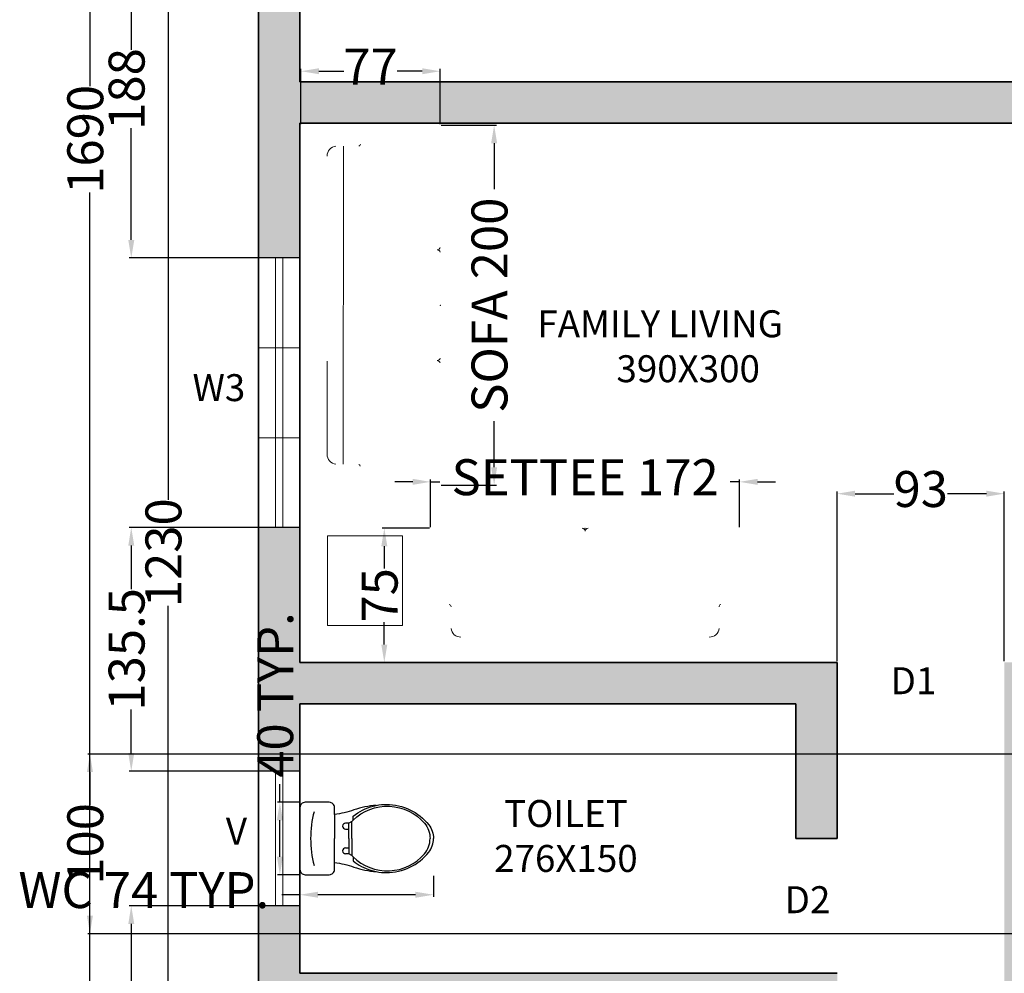
# Model space of a CAD drawing. Units: centimetres. Extents: x 2137 to 3697, y 183 to 2094.
# Tile 2 of 8: x 2137 to 2685, y 678 to 1208. Entities that reach past the tile are written whole.
import ezdxf

# ---------------------------------------------------------------- set-up
doc = ezdxf.new("R2010")
doc.units = ezdxf.units.CM
for name, color, linetype, lineweight in [('A-ANNO-DIMS', 2, 'Continuous', 18), ('A-ANNO-TEXT', 7, 'Continuous', 18), ('A-AREA-IDEN', 7, 'Continuous', 25), ('A-FLOR-FIXT', 71, 'Continuous', 18), ('A-FURN', 8, 'Continuous', 18), ('A-GLAZ', 4, 'Continuous', 18), ('A-WALL', 7, 'Continuous', 35), ('A-WALL-PATT', 52, 'Continuous', 13)]:
    doc.layers.add(name, color=color, linetype=linetype, lineweight=lineweight)
doc.layers.add('WC-Detail_dwgmodels.com', color=251, linetype='Continuous')
doc.layers.add('WC-Outline_dwgmodels.com', color=250, linetype='Continuous')
doc.styles.get("Standard").update_dxf_attribs({"font": 'arial.ttf'})
doc.dimstyles.new('ISO-25', dxfattribs={"dimtxt": 20, "dimasz": 10, "dimexe": 1.25, "dimexo": 0.625, "dimtad": 0, "dimtxsty": 'Standard', "dimcen": 2.5, "dimadec": 0, "dimazin": 0, "dimtfac": 1, "dimtmove": 0, "dimatfit": 3, "dimfxl": 1, "dimarcsym": 0})

# ---------------------------------------------------------------- blocks, each defined once
blk = doc.blocks.new('*D7')
at = {"layer": 'A-ANNO-DIMS', "color": 0, "lineweight": -2, "transparency": 16777216}
for p, q in [((2269.4, 1526.58), (2218.41, 1526.58)), ((2219.66, 1516.58), (2219.66, 941.09)), ((2219.66, 306.58), (2219.66, 882.07)), ((2269.4, 296.58), (2218.41, 296.58))]:
    blk.add_line(p, q, dxfattribs=at)
at = {"layer": 'A-ANNO-DIMS', "color": 0, "transparency": 16777216}
for points in [[(2217.99, 1516.58), (2221.33, 1516.58), (2219.66, 1526.58)], [(2217.99, 306.58), (2221.33, 306.58), (2219.66, 296.58)]]:
    blk.add_solid(points, dxfattribs=at)
at = {"layer": 'Defpoints', "color": 0, "transparency": 16777216}
for p in [(2270.02, 1526.58), (2219.66, 296.58), (2270.02, 296.58)]:
    blk.add_point(p, dxfattribs=at)
at = {"layer": 'A-ANNO-DIMS', "color": 0, "transparency": 16777216, "insert": (2219.66, 911.58), "char_height": 20, "attachment_point": 5, "rotation": 90}
blk.add_mtext('1230', dxfattribs=at)
blk = doc.blocks.new('PAN')
at = {"layer": 'WC-Detail_dwgmodels.com'}
for p, q in [((3002.19, 2116.71), (3003.1, 2118.39)), ((3003.1, 2118.39), (3003.1, 2120.22)), ((3006.38, 2118.39), (3003.1, 2118.39)), ((3006.38, 2120.22), (3006.38, 2118.39)), ((3011.63, 2118.39), (3006.38, 2118.39)), ((3011.63, 2118.39), (3016.89, 2118.39)), ((3016.89, 2120.22), (3016.89, 2118.39)), ((3016.89, 2118.39), (3020.16, 2118.39)), ((3020.16, 2118.39), (3020.16, 2120.22)), ((3021.08, 2116.71), (3020.16, 2118.39))]:
    blk.add_line(p, q, dxfattribs=at)
for points in [[(3001.49, 2116.03, 0.434217), (3003.1, 2076.32, 0.182634), (3011.63, 2073.2, 2.693815)], [(2999.21, 2116.03, 0.094048), (2994, 2106.21, 0.16845)], [(3001.49, 2116.03), (2999.21, 2116.03, 0.416606)], [(3002.19, 2116.71, 0.008985), (3001.49, 2116.03, 0.182634)], [(3011.63, 2116.71), (3002.19, 2116.71, 0.008985)], [(3011.63, 2116.71), (3021.08, 2116.71, -0.444938)], [(3021.78, 2116.03, -0.434217), (3020.16, 2076.32, -0.182634), (3011.63, 2073.2, -2.693815)], [(3021.08, 2116.71, -0.008985), (3021.78, 2116.03, -0.182634)], [(3021.78, 2116.03), (3024.05, 2116.03, -0.416606)], [(3024.05, 2116.03, -0.105447), (3029.64, 2104.91, -0.16845)], [(2994, 2106.21, 0.026594), (2993.22, 2103.13, 0.16845)], [(3029.64, 2104.91, -0.015301), (3030.05, 2103.13, -0.16845)]]:
    blk.add_lwpolyline(points, format="xyb", dxfattribs=at)
for centre, radius, start, end in [((3011.66, 2080.58), 59.08, 90.028, 104.6712), ((3011.6, 2080.58), 59.08, 75.3288, 89.972), ((3004.74, 2120.22), 1.64, 0, 180), ((3018.53, 2120.22), 1.64, 0, 180)]:
    blk.add_arc(centre, radius, start, end, dxfattribs=at)
at = {"layer": 'WC-Outline_dwgmodels.com'}
for points in [[(3028.88, 2126.37, 0.414214), (3031.77, 2129.26), (3031.77, 2142.74, 0.414214), (3028.88, 2145.63), (3011.63, 2145.63), (2994.39, 2145.63, 0.414214), (2991.49, 2142.74), (2991.49, 2129.26, 0.414214), (2994.39, 2126.37), (2998.34, 2126.37, -0.052345), (2995.73, 2115.59, 0.071131), (2993.22, 2103.13, 0.160777)], [(2998.34, 2126.37), (3011.63, 2126.37, 0.414214)], [(3024.93, 2126.37), (3011.63, 2126.37, -0.414214)], [(3030.05, 2103.13, 0.071131), (3027.53, 2115.59, -0.052345), (3024.93, 2126.37), (3028.88, 2126.37, 0.414214)], [(2993.22, 2103.13, 0.048023), (2992.66, 2097.45, 0.16845)], [(3030.05, 2103.13, -0.048023), (3030.61, 2097.45, -0.16845)], [(2992.66, 2097.45, 0.230343), (3004.02, 2073.95, 0.16845), (3011.63, 2071.31, 2.883082)], [(3030.61, 2097.45, -0.230343), (3019.25, 2073.95, -0.16845), (3011.63, 2071.31, -2.883082)]]:
    blk.add_lwpolyline(points, format="xyb", dxfattribs=at)
blk = doc.blocks.new('Clinicians and patient chairs 9_dwgmodels.com')
at = {"color": 0}
for points in [[(-907.9, 0, 0, 0, 0), (-959.6, -11.1, 4.62, 4.62, 0)], [(907.9, 0, 0, 0, 0), (-907.9, 0, 4.62, 4.62, 0)], [(959.6, -11.1, 0, 0, 0), (907.9, 0, 4.62, 4.62, 0)], [(-994.7, -35.9, 0, 0, 0), (-1015.6, -68.3, 4.62, 4.62, 0)], [(-959.6, -11.1, 0, 0, 0), (-994.7, -35.9, 4.62, 4.62, 0)], [(994.7, -35.9, 0, 0, 0), (959.6, -11.1, 4.62, 4.62, 0)], [(1015.6, -68.3, 0, 0, 0), (994.7, -35.9, 4.62, 4.62, 0)], [(-1015.6, -68.3, 0, 0, 0), (-1025.5, -106.3, 4.62, 4.62, 0)], [(-1025.5, -106.3, 0, 0, 0), (-1025.5, -779.5, 4.62, 4.62, 0)], [(1025.5, -106.3, 0, 0, 0), (1015.6, -68.3, 4.62, 4.62, 0)], [(1025.5, -779.5, 0, 0, 0), (1025.5, -106.3, 4.62, 4.62, 0)], [(-313.4, -149.9, 0, 0, 0), (-318.1, -149.9, 4.62, 4.62, 0)], [(-314.5, -150.4, 0, 0, 0), (-315.7, -159.3, 4.62, 4.62, 0)], [(-315.7, -159.3, 0, 0, 0), (-315.7, -777.3, 4.62, 4.62, 0)], [(-309.5, -148.3, 0, 0, 0), (-314.5, -150.4, 4.62, 4.62, 0)], [(-308, -148.3, 0, 0, 0), (-309.5, -148.3, 4.62, 4.62, 0)], [(-307.5, -148.3, 0, 0, 0), (-308, -148.3, 4.62, 4.62, 0)], [(242.9, -148.3, 0, 0, 0), (-307.5, -148.3, 4.62, 4.62, 0)], [(242.9, -148.3, 0, 0, 0), (296, -148.3, 4.62, 4.62, 0)], [(296, -148.3, 0, 0, 0), (307.5, -148.3, 4.62, 4.62, 0)], [(308, -148.3, 0, 0, 0), (307.5, -148.3, 4.62, 4.62, 0)], [(309.5, -148.3, 0, 0, 0), (308, -148.3, 4.62, 4.62, 0)], [(309.5, -148.3, 0, 0, 0), (314.5, -150.4, 4.62, 4.62, 0)], [(849.5, -149.9, 0, 0, 0), (313.4, -149.9, 4.62, 4.62, 0)], [(314.5, -150.4, 0, 0, 0), (315.7, -159.3, 4.62, 4.62, 0)], [(315.7, -159.3, 0, 0, 0), (315.7, -777.3, 4.62, 4.62, 0)], [(315.7, -161.8, 0, 0, 0), (315.7, -777.3, 4.62, 4.62, 0)], [(1025.5, -779.5, 0, 0, 0), (1025.5, -117.3, 4.62, 4.62, 0)], [(-906.6, -285, 0, 0, 0), (-906.4, -198.1, 4.62, 4.62, 0)], [(906.9, -327, 0, 0, 0), (906.4, -199.7, 4.62, 4.62, 0)], [(-1023, -329.7, 0, 0, 0), (-1019.2, -332.9, 4.62, 4.62, 0)], [(-1010.3, -335.9, 0, 0, 0), (-1019.8, -340.2, 4.62, 4.62, 0)], [(-1019.2, -332.9, 0, 0, 0), (-1019, -333, 4.62, 4.62, 0)], [(-1019, -333, 0, 0, 0), (-1018.9, -333.1, 4.62, 4.62, 0)], [(-1013.9, -334.2, 0, 0, 0), (-1018.9, -333.1, 4.62, 4.62, 0)], [(-1013.9, -334.2, 0, 0, 0), (-964.4, -335.7, 4.62, 4.62, 0)], [(-917.1, -337, 0, 0, 0), (-1010.3, -335.9, 4.62, 4.62, 0)], [(-964.4, -335.7, 0, 0, 0), (-927.1, -336.8, 4.62, 4.62, 0)], [(-906.8, -305.4, 0, 0, 0), (-906.9, -324.5, 4.62, 4.62, 0)], [(-906.9, -324.5, 0, 0, 0), (-906.9, -329.8, 4.62, 4.62, 0)], [(-906.6, -285, 0, 0, 0), (-906.8, -305.4, 4.62, 4.62, 0)], [(906.9, -327, 0, 0, 0), (906.9, -329.9, 4.62, 4.62, 0)], [(964.4, -335.7, 0, 0, 0), (914.9, -337.2, 4.62, 4.62, 0)], [(917.1, -339.4, 0, 0, 0), (1010.3, -338.4, 4.62, 4.62, 0)], [(1013.9, -334.2, 0, 0, 0), (964.4, -335.7, 4.62, 4.62, 0)], [(1010.3, -338.4, 0, 0, 0), (1019.8, -342.7, 4.62, 4.62, 0)], [(1013.9, -334.2, 0, 0, 0), (1018.9, -333.1, 4.62, 4.62, 0)], [(1018.9, -333.1, 0, 0, 0), (1019, -333, 4.62, 4.62, 0)], [(1019.2, -332.9, 0, 0, 0), (1019, -333, 4.62, 4.62, 0)], [(1023, -329.7, 0, 0, 0), (1019.2, -332.9, 4.62, 4.62, 0)], [(-1019.8, -340.2, 0, 0, 0), (-1023, -348.6, 4.62, 4.62, 0)], [(1019.8, -342.7, 0, 0, 0), (1023, -351.1, 4.62, 4.62, 0)], [(1023, -351.1, 0, 0, 0), (1022.6, -779.8, 4.62, 4.62, 0)], [(-1025.5, -779.5, 0, 0, 0), (-1022.2, -788.7, 4.62, 4.62, 0)], [(1022.6, -779.8, 0, 0, 0), (1019.8, -788.8, 4.62, 4.62, 0)], [(1022.2, -788.7, 0, 0, 0), (1025.5, -779.5, 4.62, 4.62, 0)], [(-1022.2, -788.7, 0, 0, 0), (-1021.6, -789.8, 4.62, 4.62, 0)], [(-1021.6, -789.8, 0, 0, 0), (-1020.6, -790.5, 4.62, 4.62, 0)], [(-1020.6, -790.5, 0, 0, 0), (-1013.6, -793.7, 4.62, 4.62, 0)], [(-1013.6, -793.7, 0, 0, 0), (1013.6, -793.7, 4.62, 4.62, 0)], [(1019.8, -788.8, 0, 0, 0), (1013.1, -793.7, 4.62, 4.62, 0)], [(1013.6, -793.7, 0, 0, 0), (1020.6, -790.5, 4.62, 4.62, 0)], [(1020.6, -790.5, 0, 0, 0), (1021.6, -789.8, 4.62, 4.62, 0)], [(1022.2, -788.7, 0, 0, 0), (1021.6, -789.8, 4.62, 4.62, 0)]]:
    blk.add_lwpolyline(points, format="xyseb", dxfattribs=at)
for points in [[(-849.5, -149.9), (-318.1, -149.9)], [(-906.5, -241.5), (906.5, -242.3)]]:
    blk.add_lwpolyline(points, dxfattribs=at)
for centre, radius, start, end in [((-851.7, -204.8), 54.9, 87.6679, 174.7256), ((851.7, -204.8), 54.9, 5.2744, 92.3321), ((-916.6, -326.8), 10.2, 267.5454, 342.4057), ((916.9, -329.4), 10, 182.6094, 270.795), ((-337, -773.8), 21.5, 292.115, 350.6304), ((-294.5, -773.8), 21.5, 189.3696, 247.885), ((294.5, -773.8), 21.5, 292.115, 350.6304), ((336.9, -773.8), 21.5, 189.3696, 247.885)]:
    blk.add_arc(centre, radius, start, end, dxfattribs=at)
blk.add_point((0, -793.7), dxfattribs=at)
blk = doc.blocks.new('Clinicians and patient chairs 13_dwgmodels.com')
at = {"color": 0}
for points in [[(-780.9, 0, 0, 0, 0), (-832.6, -11.1, 4.5, 4.5, 0)], [(-780.8, -0.7, 0, 0, 0), (-832.3, -11.8, 4.5, 4.5, 0)], [(-780.8, -0.7, 0, 0, 0), (-832.3, -11.8, 4.5, 4.5, 0)], [(780.9, 0, 0, 0, 0), (-780.9, 0, 4.5, 4.5, 0)], [(780.8, -0.7, 0, 0, 0), (-780.8, -0.7, 4.5, 4.5, 0)], [(780.8, -0.7, 0, 0, 0), (-780.8, -0.7, 4.5, 4.5, 0)], [(832.3, -11.8, 0, 0, 0), (780.8, -0.7, 4.5, 4.5, 0)], [(832.3, -11.8, 0, 0, 0), (780.8, -0.7, 4.5, 4.5, 0)], [(832.6, -11.1, 0, 0, 0), (780.9, 0, 4.5, 4.5, 0)], [(-867.7, -35.9, 0, 0, 0), (-888.6, -68.3, 4.5, 4.5, 0)], [(-867.1, -36.4, 0, 0, 0), (-888, -68.6, 4.5, 4.5, 0)], [(-867.1, -36.4, 0, 0, 0), (-888, -68.6, 4.5, 4.5, 0)], [(-872.1, -47.4, 0, 0, 0), (-872.1, -47.3, 4.5, 4.5, 0)], [(-832.6, -11.1, 0, 0, 0), (-867.7, -35.9, 4.5, 4.5, 0)], [(-832.3, -11.8, 0, 0, 0), (-867.1, -36.4, 4.5, 4.5, 0)], [(-832.3, -11.8, 0, 0, 0), (-867.1, -36.4, 4.5, 4.5, 0)], [(-854.1, -29.4, 0, 0, 0), (-854.1, -29.4, 4.5, 4.5, 0)], [(867.1, -36.4, 0, 0, 0), (832.3, -11.8, 4.5, 4.5, 0)], [(867.1, -36.4, 0, 0, 0), (832.3, -11.8, 4.5, 4.5, 0)], [(867.7, -35.9, 0, 0, 0), (832.6, -11.1, 4.5, 4.5, 0)], [(888, -68.6, 0, 0, 0), (867.1, -36.4, 4.5, 4.5, 0)], [(888, -68.6, 0, 0, 0), (867.1, -36.4, 4.5, 4.5, 0)], [(888.6, -68.3, 0, 0, 0), (867.7, -35.9, 4.5, 4.5, 0)], [(-888.6, -68.3, 0, 0, 0), (-898.5, -106.3, 4.5, 4.5, 0)], [(-898.5, -106.3, 0, 0, 0), (-898.5, -766.8, 4.5, 4.5, 0)], [(-888, -68.6, 0, 0, 0), (-897.8, -106.4, 4.5, 4.5, 0)], [(-897.8, -106.4, 0, 0, 0), (-897.8, -114.4, 4.5, 4.5, 0)], [(-897.8, -106.4, 0, 0, 0), (-897.8, -114.4, 4.5, 4.5, 0)], [(-897.8, -114.4, 0, 0, 0), (-897.8, -766.7, 4.5, 4.5, 0)], [(-897.8, -114.4, 0, 0, 0), (-897.8, -766.7, 4.5, 4.5, 0)], [(-897.8, -766.7, 0, 0, 0), (-897.8, -114.4, 4.5, 4.5, 0)], [(897.8, -106.4, 0, 0, 0), (888, -68.6, 4.5, 4.5, 0)], [(897.8, -106.4, 0, 0, 0), (888, -68.6, 4.5, 4.5, 0)], [(898.5, -106.3, 0, 0, 0), (888.6, -68.3, 4.5, 4.5, 0)], [(897.8, -114.4, 0, 0, 0), (897.8, -106.4, 4.5, 4.5, 0)], [(897.8, -114.4, 0, 0, 0), (897.8, -106.4, 4.5, 4.5, 0)], [(897.8, -766.7, 0, 0, 0), (897.8, -114.4, 4.5, 4.5, 0)], [(898.5, -766.8, 0, 0, 0), (898.5, -106.3, 4.5, 4.5, 0)], [(-896, -117.6, 0, 0, 0), (-896, -126.8, 4.5, 4.5, 0)], [(-896, -117.6, 0, 0, 0), (-896, -324.6, 4.5, 4.5, 0)], [(-896, -126.8, 0, 0, 0), (-896, -324.6, 4.5, 4.5, 0)], [(-22.2, -148.3, 0, 0, 0), (-722.5, -148.3, 4.5, 4.5, 0)], [(-8.3, -148.3, 0, 0, 0), (-22.2, -148.3, 4.5, 4.5, 0)], [(-8.3, -148.3, 0, 0, 0), (-7.7, -148.3, 4.5, 4.5, 0)], [(-7.7, -148.3, 0, 0, 0), (-6.2, -148.3, 4.5, 4.5, 0)], [(-6.2, -148.3, 0, 0, 0), (-1.3, -150.4, 4.5, 4.5, 0)], [(2.3, -149.9, 0, 0, 0), (-2.3, -149.9, 4.5, 4.5, 0)], [(-1.3, -150.4, 0, 0, 0), (0, -159.3, 4.5, 4.5, 0)], [(1.3, -150.4, 0, 0, 0), (0, -159.3, 4.5, 4.5, 0)], [(0, -159.3, 0, 0, 0), (0, -764.6, 4.5, 4.5, 0)], [(0, -159.3, 0, 0, 0), (0, -764.6, 4.5, 4.5, 0)], [(6.2, -148.3, 0, 0, 0), (1.3, -150.4, 4.5, 4.5, 0)], [(7.7, -148.3, 0, 0, 0), (6.2, -148.3, 4.5, 4.5, 0)], [(8.3, -148.3, 0, 0, 0), (7.7, -148.3, 4.5, 4.5, 0)], [(22.2, -148.3, 0, 0, 0), (8.3, -148.3, 4.5, 4.5, 0)], [(206.6, -148.3, 0, 0, 0), (22.2, -148.3, 4.5, 4.5, 0)], [(206.6, -148.3, 0, 0, 0), (722.5, -148.3, 4.5, 4.5, 0)], [(898.5, -766.8, 0, 0, 0), (898.5, -117.3, 4.5, 4.5, 0)], [(-779.6, -285, 0, 0, 0), (-779.4, -198.1, 4.5, 4.5, 0)], [(779.6, -285, 0, 0, 0), (779.4, -198.1, 4.5, 4.5, 0)], [(-896, -321.9, 0, 0, 0), (-896, -251.5, 4.5, 4.5, 0)], [(-779.6, -285, 0, 0, 0), (-779.8, -305.4, 4.5, 4.5, 0)], [(779.6, -285, 0, 0, 0), (779.8, -305.4, 4.5, 4.5, 0)], [(-896, -317.7, 0, 0, 0), (-896, -329.7, 4.5, 4.5, 0)], [(-896, -320.4, 0, 0, 0), (-896, -324.6, 4.5, 4.5, 0)], [(-896, -321.9, 0, 0, 0), (-896, -329.7, 4.5, 4.5, 0)], [(-896, -329.7, 0, 0, 0), (-896, -321.9, 4.5, 4.5, 0)], [(-896, -329.7, 0, 0, 0), (-892.2, -332.9, 4.5, 4.5, 0)], [(-892.2, -332.9, 0, 0, 0), (-892, -333, 4.5, 4.5, 0)], [(-892, -333, 0, 0, 0), (-891.9, -333.1, 4.5, 4.5, 0)], [(-886.9, -334.2, 0, 0, 0), (-891.9, -333.1, 4.5, 4.5, 0)], [(-886.9, -334.2, 0, 0, 0), (-837.4, -335.7, 4.5, 4.5, 0)], [(-837.4, -335.7, 0, 0, 0), (-790.1, -337, 4.5, 4.5, 0)], [(-779.8, -305.4, 0, 0, 0), (-779.9, -324.5, 4.5, 4.5, 0)], [(779.8, -305.4, 0, 0, 0), (779.9, -324.5, 4.5, 4.5, 0)], [(837.4, -335.7, 0, 0, 0), (790.1, -337, 4.5, 4.5, 0)], [(886.9, -334.2, 0, 0, 0), (837.4, -335.7, 4.5, 4.5, 0)], [(886.9, -334.2, 0, 0, 0), (891.9, -333.1, 4.5, 4.5, 0)], [(891.9, -333.1, 0, 0, 0), (892, -333, 4.5, 4.5, 0)], [(892.2, -332.9, 0, 0, 0), (892, -333, 4.5, 4.5, 0)], [(896, -329.7, 0, 0, 0), (892.2, -332.9, 4.5, 4.5, 0)], [(-898.5, -766.8, 0, 0, 0), (-895.2, -776, 4.5, 4.5, 0)], [(-895.2, -776, 0, 0, 0), (-898.5, -766.8, 4.5, 4.5, 0)], [(-897.8, -766.7, 0, 0, 0), (-894.5, -775.7, 4.5, 4.5, 0)], [(-897.8, -766.7, 0, 0, 0), (-894.5, -775.7, 4.5, 4.5, 0)], [(-894.5, -775.7, 0, 0, 0), (-897.8, -766.7, 4.5, 4.5, 0)], [(-894.5, -775.7, 0, 0, 0), (-897.8, -766.7, 4.5, 4.5, 0)], [(-895.2, -776, 0, 0, 0), (-894.6, -777.1, 4.5, 4.5, 0)], [(-894.6, -777.1, 0, 0, 0), (-895.2, -776, 4.5, 4.5, 0)], [(-894.5, -775.7, 0, 0, 0), (-894, -776.6, 4.5, 4.5, 0)], [(-894.5, -775.7, 0, 0, 0), (-894, -776.6, 4.5, 4.5, 0)], [(-894, -776.6, 0, 0, 0), (-894.5, -775.7, 4.5, 4.5, 0)], [(-894, -776.6, 0, 0, 0), (-894.5, -775.7, 4.5, 4.5, 0)], [(-894.6, -777.1, 0, 0, 0), (-893.6, -777.8, 4.5, 4.5, 0)], [(-893.6, -777.8, 0, 0, 0), (-894.6, -777.1, 4.5, 4.5, 0)], [(-894, -776.6, 0, 0, 0), (-893.2, -777.2, 4.5, 4.5, 0)], [(-894, -776.6, 0, 0, 0), (-893.2, -777.2, 4.5, 4.5, 0)], [(-893.2, -777.2, 0, 0, 0), (-894, -776.6, 4.5, 4.5, 0)], [(-893.2, -777.2, 0, 0, 0), (-894, -776.6, 4.5, 4.5, 0)], [(-893.6, -777.8, 0, 0, 0), (-886.6, -781, 4.5, 4.5, 0)], [(-886.6, -781, 0, 0, 0), (-893.6, -777.8, 4.5, 4.5, 0)], [(-893.2, -777.2, 0, 0, 0), (-886.5, -780.3, 4.5, 4.5, 0)], [(-893.2, -777.2, 0, 0, 0), (-886.5, -780.3, 4.5, 4.5, 0)], [(-886.5, -780.3, 0, 0, 0), (-893.2, -777.2, 4.5, 4.5, 0)], [(-886.5, -780.3, 0, 0, 0), (-893.2, -777.2, 4.5, 4.5, 0)], [(-886.6, -781, 0, 0, 0), (886.6, -781, 4.5, 4.5, 0)], [(886.6, -781, 0, 0, 0), (-886.6, -781, 4.5, 4.5, 0)], [(-886.5, -780.3, 0, 0, 0), (886.5, -780.3, 4.5, 4.5, 0)], [(-886.5, -780.3, 0, 0, 0), (886.5, -780.3, 4.5, 4.5, 0)], [(886.5, -780.3, 0, 0, 0), (-886.5, -780.3, 4.5, 4.5, 0)], [(886.5, -780.3, 0, 0, 0), (-886.5, -780.3, 4.5, 4.5, 0)], [(886.5, -780.3, 0, 0, 0), (893.2, -777.2, 4.5, 4.5, 0)], [(886.5, -780.3, 0, 0, 0), (893.2, -777.2, 4.5, 4.5, 0)], [(893.2, -777.2, 0, 0, 0), (886.5, -780.3, 4.5, 4.5, 0)], [(893.2, -777.2, 0, 0, 0), (886.5, -780.3, 4.5, 4.5, 0)], [(886.6, -781, 0, 0, 0), (893.6, -777.8, 4.5, 4.5, 0)], [(893.6, -777.8, 0, 0, 0), (886.6, -781, 4.5, 4.5, 0)], [(893.2, -777.2, 0, 0, 0), (894, -776.6, 4.5, 4.5, 0)], [(893.2, -777.2, 0, 0, 0), (894, -776.6, 4.5, 4.5, 0)], [(894, -776.6, 0, 0, 0), (893.2, -777.2, 4.5, 4.5, 0)], [(894, -776.6, 0, 0, 0), (893.2, -777.2, 4.5, 4.5, 0)], [(893.6, -777.8, 0, 0, 0), (894.6, -777.1, 4.5, 4.5, 0)], [(894.6, -777.1, 0, 0, 0), (893.6, -777.8, 4.5, 4.5, 0)], [(894.5, -775.7, 0, 0, 0), (894, -776.6, 4.5, 4.5, 0)], [(894.5, -775.7, 0, 0, 0), (894, -776.6, 4.5, 4.5, 0)], [(894.5, -775.7, 0, 0, 0), (894, -776.6, 4.5, 4.5, 0)], [(894.5, -775.7, 0, 0, 0), (894, -776.6, 4.5, 4.5, 0)], [(894.5, -775.7, 0, 0, 0), (897.8, -766.7, 4.5, 4.5, 0)], [(894.5, -775.7, 0, 0, 0), (897.8, -766.7, 4.5, 4.5, 0)], [(897.8, -766.7, 0, 0, 0), (894.5, -775.7, 4.5, 4.5, 0)], [(897.8, -766.7, 0, 0, 0), (894.5, -775.7, 4.5, 4.5, 0)], [(895.2, -776, 0, 0, 0), (894.6, -777.1, 4.5, 4.5, 0)], [(895.2, -776, 0, 0, 0), (894.6, -777.1, 4.5, 4.5, 0)], [(895.2, -776, 0, 0, 0), (898.5, -766.8, 4.5, 4.5, 0)], [(898.5, -766.8, 0, 0, 0), (895.2, -776, 4.5, 4.5, 0)]]:
    blk.add_lwpolyline(points, format="xyseb", dxfattribs=at)
for points in [[(-779.9, -324.5), (-779.9, -328.3)], [(779.9, -324.5), (779.9, -325.8)]]:
    blk.add_lwpolyline(points, dxfattribs=at)
for centre, radius, start, end in [((-724.7, -203.1), 54.9, 87.6679, 174.7255), ((724.7, -203.1), 54.9, 5.2744, 92.3321), ((-789.7, -327.1), 9.9, 267.955, 352.9309), ((791.8, -325.1), 12, 183.2786, 261.4861), ((-17.2, -763), 17.3, 271.1045, 354.6239), ((17.2, -763), 17.3, 185.3761, 268.8955)]:
    blk.add_arc(centre, radius, start, end, dxfattribs=at)
blk.add_point((0, -781), dxfattribs=at)
blk = doc.blocks.new('WIN-W3-150CM')
for p, q in [((0, 23), (0, 0)), ((50, 23), (50, 0)), ((100, 23), (100, 0)), ((150, 23), (150, 0)), ((0, 13.5), (150, 13.5)), ((0, 9.5), (150, 9.5))]:
    blk.add_line(p, q)
blk = doc.blocks.new('VENT-75CM')
for p, q in [((0, 0), (0, 23)), ((75, 0), (75, 23)), ((0, 13.5), (75, 13.5)), ((0, 9.5), (75, 9.5))]:
    blk.add_line(p, q)
blk = doc.blocks.new('*D24')
at = {"layer": 'A-ANNO-DIMS', "color": 0, "lineweight": -2, "transparency": 16777216}
for p, q in [((2293.02, 731.82), (2293.02, 720.04)), ((2367.34, 731.82), (2367.34, 720.04)), ((2293.02, 721.29), (2283.02, 721.29)), ((2357.34, 721.29), (2303.02, 721.29))]:
    blk.add_line(p, q, dxfattribs=at)
at = {"layer": 'A-ANNO-DIMS', "color": 0, "transparency": 16777216}
for points in [[(2303.02, 722.96), (2303.02, 719.63), (2293.02, 721.29)], [(2357.34, 722.96), (2357.34, 719.63), (2367.34, 721.29)]]:
    blk.add_solid(points, dxfattribs=at)
at = {"layer": 'Defpoints', "color": 0, "transparency": 16777216}
for p in [(2293.02, 732.44), (2367.34, 732.44), (2293.02, 721.29)]:
    blk.add_point(p, dxfattribs=at)
at = {"layer": 'A-ANNO-DIMS', "color": 0, "transparency": 16777216, "insert": (2206.16, 721.29), "char_height": 20, "attachment_point": 5}
blk.add_mtext('WC 74 TYP.', dxfattribs=at)
blk = doc.blocks.new('*D25')
at = {"layer": 'A-ANNO-DIMS', "color": 0, "lineweight": -2, "transparency": 16777216}
for p, q in [((2281.87, 772.72), (2281.87, 782.72)), ((2292.4, 772.72), (2280.62, 772.72)), ((2281.87, 742.44), (2281.87, 762.72)), ((2292.4, 732.44), (2280.62, 732.44))]:
    blk.add_line(p, q, dxfattribs=at)
at = {"layer": 'A-ANNO-DIMS', "color": 0, "transparency": 16777216}
for points in [[(2280.21, 762.72), (2283.54, 762.72), (2281.87, 772.72)], [(2280.21, 742.44), (2283.54, 742.44), (2281.87, 732.44)]]:
    blk.add_solid(points, dxfattribs=at)
at = {"layer": 'Defpoints', "color": 0, "transparency": 16777216}
for p in [(2281.87, 772.72), (2293.02, 772.72), (2293.02, 732.44)]:
    blk.add_point(p, dxfattribs=at)
at = {"layer": 'A-ANNO-DIMS', "color": 0, "transparency": 16777216, "insert": (2281.87, 832.42), "char_height": 20, "attachment_point": 5, "rotation": 90}
blk.add_mtext('40 TYP.', dxfattribs=at)
blk = doc.blocks.new('*D32')
at = {"layer": 'A-ANNO-DIMS', "color": 0, "lineweight": -2, "transparency": 16777216}
for p, q in [((2371.71, 1149.44), (2402.37, 1149.44)), ((2401.12, 1139.44), (2401.12, 1113.86)), ((2401.12, 959.18), (2401.12, 984.75)), ((2371.71, 949.18), (2402.37, 949.18))]:
    blk.add_line(p, q, dxfattribs=at)
at = {"layer": 'A-ANNO-DIMS', "color": 0, "transparency": 16777216}
for points in [[(2399.45, 1139.44), (2402.79, 1139.44), (2401.12, 1149.44)], [(2399.45, 959.18), (2402.79, 959.18), (2401.12, 949.18)]]:
    blk.add_solid(points, dxfattribs=at)
at = {"layer": 'Defpoints', "color": 0, "transparency": 16777216}
for p in [(2371.08, 1149.44), (2401.12, 1149.44), (2371.08, 949.18)]:
    blk.add_point(p, dxfattribs=at)
at = {"layer": 'A-ANNO-DIMS', "color": 0, "transparency": 16777216, "insert": (2401.12, 1049.31), "char_height": 20, "attachment_point": 5, "rotation": 90}
blk.add_mtext('SOFA 200', dxfattribs=at)
blk = doc.blocks.new('*D33')
at = {"layer": 'A-ANNO-DIMS', "color": 0, "lineweight": -2, "transparency": 16777216}
for p, q in [((2293.58, 1150.06), (2293.58, 1180.73)), ((2303.58, 1179.48), (2317.46, 1179.48)), ((2361.08, 1179.48), (2347.2, 1179.48)), ((2371.08, 1150.06), (2371.08, 1180.73))]:
    blk.add_line(p, q, dxfattribs=at)
at = {"layer": 'A-ANNO-DIMS', "color": 0, "transparency": 16777216}
for points in [[(2303.58, 1181.14), (2303.58, 1177.81), (2293.58, 1179.48)], [(2361.08, 1181.14), (2361.08, 1177.81), (2371.08, 1179.48)]]:
    blk.add_solid(points, dxfattribs=at)
at = {"layer": 'Defpoints', "color": 0, "transparency": 16777216}
for p in [(2293.58, 1179.48), (2293.58, 1149.44), (2371.08, 1149.44)]:
    blk.add_point(p, dxfattribs=at)
at = {"layer": 'A-ANNO-DIMS', "color": 0, "transparency": 16777216, "insert": (2332.33, 1179.48), "char_height": 20, "attachment_point": 5}
blk.add_mtext('77', dxfattribs=at)
blk = doc.blocks.new('*D34')
at = {"layer": 'A-ANNO-DIMS', "color": 0, "lineweight": -2, "transparency": 16777216}
for p, q in [((2355.78, 951.01), (2345.78, 951.01)), ((2365.78, 925.85), (2365.78, 952.26)), ((2365.78, 951.01), (2370.95, 951.01)), ((2537.69, 951.01), (2532.53, 951.01)), ((2537.69, 925.85), (2537.69, 952.26)), ((2547.69, 951.01), (2557.69, 951.01))]:
    blk.add_line(p, q, dxfattribs=at)
at = {"layer": 'A-ANNO-DIMS', "color": 0, "transparency": 16777216}
for points in [[(2355.78, 952.68), (2355.78, 949.35), (2365.78, 951.01)], [(2547.69, 952.68), (2547.69, 949.35), (2537.69, 951.01)]]:
    blk.add_solid(points, dxfattribs=at)
at = {"layer": 'Defpoints', "color": 0, "transparency": 16777216}
for p in [(2365.78, 951.01), (2365.78, 925.23), (2537.69, 925.23)]:
    blk.add_point(p, dxfattribs=at)
at = {"layer": 'A-ANNO-DIMS', "color": 0, "transparency": 16777216, "insert": (2451.74, 951.01), "char_height": 20, "attachment_point": 5}
blk.add_mtext('SETTEE 172', dxfattribs=at)
blk = doc.blocks.new('*D35')
at = {"layer": 'A-ANNO-DIMS', "color": 0, "lineweight": -2, "transparency": 16777216}
for p, q in [((2365.16, 925.23), (2338.74, 925.23)), ((2339.99, 915.23), (2339.99, 902.81)), ((2339.99, 860.51), (2339.99, 872.92)), ((2365.16, 850.51), (2338.74, 850.51))]:
    blk.add_line(p, q, dxfattribs=at)
at = {"layer": 'A-ANNO-DIMS', "color": 0, "transparency": 16777216}
for points in [[(2338.33, 915.23), (2341.66, 915.23), (2339.99, 925.23)], [(2338.33, 860.51), (2341.66, 860.51), (2339.99, 850.51)]]:
    blk.add_solid(points, dxfattribs=at)
at = {"layer": 'Defpoints', "color": 0, "transparency": 16777216}
for p in [(2365.78, 925.23), (2339.99, 850.51), (2365.78, 850.51)]:
    blk.add_point(p, dxfattribs=at)
at = {"layer": 'A-ANNO-DIMS', "color": 0, "transparency": 16777216, "insert": (2339.99, 887.87), "char_height": 20, "attachment_point": 5, "rotation": 90}
blk.add_mtext('75', dxfattribs=at)
blk = doc.blocks.new('*D38')
at = {"layer": 'A-ANNO-DIMS', "color": 0, "lineweight": -2, "transparency": 16777216}
for p, q in [((2857.4, 1986.58), (2174.92, 1986.58)), ((2176.17, 1976.58), (2176.17, 1171.09)), ((2176.17, 306.58), (2176.17, 1112.07)), ((2269.4, 296.58), (2174.92, 296.58))]:
    blk.add_line(p, q, dxfattribs=at)
at = {"layer": 'A-ANNO-DIMS', "color": 0, "transparency": 16777216}
for points in [[(2174.51, 1976.58), (2177.84, 1976.58), (2176.17, 1986.58)], [(2174.51, 306.58), (2177.84, 306.58), (2176.17, 296.58)]]:
    blk.add_solid(points, dxfattribs=at)
at = {"layer": 'Defpoints', "color": 0, "transparency": 16777216}
for p in [(2176.17, 1986.58), (2858.02, 1986.58), (2270.02, 296.58)]:
    blk.add_point(p, dxfattribs=at)
at = {"layer": 'A-ANNO-DIMS', "color": 0, "transparency": 16777216, "insert": (2176.17, 1141.58), "char_height": 20, "attachment_point": 5, "rotation": 90}
blk.add_mtext('1690', dxfattribs=at)
blk = doc.blocks.new('*D42')
at = {"layer": 'A-ANNO-DIMS', "color": 0, "lineweight": -2, "transparency": 16777216}
for p, q in [((3183.4, 799.58), (2174.92, 799.58)), ((2176.17, 789.58), (2176.17, 771.32)), ((2176.17, 709.58), (2176.17, 727.84)), ((3183.4, 699.58), (2174.92, 699.58))]:
    blk.add_line(p, q, dxfattribs=at)
at = {"layer": 'A-ANNO-DIMS', "color": 0, "transparency": 16777216}
for points in [[(2174.51, 789.58), (2177.84, 789.58), (2176.17, 799.58)], [(2174.51, 709.58), (2177.84, 709.58), (2176.17, 699.58)]]:
    blk.add_solid(points, dxfattribs=at)
at = {"layer": 'Defpoints', "color": 0, "transparency": 16777216}
for p in [(2176.17, 799.58), (3184.02, 799.58), (3184.02, 699.58)]:
    blk.add_point(p, dxfattribs=at)
at = {"layer": 'A-ANNO-DIMS', "color": 0, "transparency": 16777216, "insert": (2176.17, 749.58), "char_height": 20, "attachment_point": 5, "rotation": 90}
blk.add_mtext('100', dxfattribs=at)
blk = doc.blocks.new('*D50')
at = {"layer": 'A-ANNO-DIMS', "color": 0, "lineweight": -2, "transparency": 16777216}
for p, q in [((2292.4, 715.08), (2197.92, 715.08)), ((2199.17, 705.08), (2199.17, 660.36)), ((2199.17, 572.08), (2199.17, 616.8)), ((2292.4, 562.08), (2197.92, 562.08))]:
    blk.add_line(p, q, dxfattribs=at)
at = {"layer": 'A-ANNO-DIMS', "color": 0, "transparency": 16777216}
for points in [[(2197.51, 705.08), (2200.84, 705.08), (2199.17, 715.08)], [(2197.51, 572.08), (2200.84, 572.08), (2199.17, 562.08)]]:
    blk.add_solid(points, dxfattribs=at)
at = {"layer": 'Defpoints', "color": 0, "transparency": 16777216}
for p in [(2199.17, 715.08), (2293.02, 715.08), (2293.02, 562.08)]:
    blk.add_point(p, dxfattribs=at)
at = {"layer": 'A-ANNO-DIMS', "color": 0, "transparency": 16777216, "insert": (2199.17, 638.58), "char_height": 20, "attachment_point": 5, "rotation": 90}
blk.add_mtext('153', dxfattribs=at)
blk = doc.blocks.new('*D51')
at = {"layer": 'A-ANNO-DIMS', "color": 0, "lineweight": -2, "transparency": 16777216}
for p, q in [((2292.4, 925.58), (2197.92, 925.58)), ((2199.17, 915.58), (2199.17, 891.33)), ((2199.17, 800.08), (2199.17, 824.33)), ((2292.4, 790.08), (2197.92, 790.08))]:
    blk.add_line(p, q, dxfattribs=at)
at = {"layer": 'A-ANNO-DIMS', "color": 0, "transparency": 16777216}
for points in [[(2197.51, 915.58), (2200.84, 915.58), (2199.17, 925.58)], [(2197.51, 800.08), (2200.84, 800.08), (2199.17, 790.08)]]:
    blk.add_solid(points, dxfattribs=at)
at = {"layer": 'Defpoints', "color": 0, "transparency": 16777216}
for p in [(2199.17, 925.58), (2293.02, 925.58), (2293.02, 790.08)]:
    blk.add_point(p, dxfattribs=at)
at = {"layer": 'A-ANNO-DIMS', "color": 0, "transparency": 16777216, "insert": (2199.17, 857.83), "char_height": 20, "attachment_point": 5, "rotation": 90}
blk.add_mtext('135.5', dxfattribs=at)
blk = doc.blocks.new('*D52')
at = {"layer": 'A-ANNO-DIMS', "color": 0, "lineweight": -2, "transparency": 16777216}
for p, q in [((2292.4, 1263.58), (2197.92, 1263.58)), ((2199.17, 1253.58), (2199.17, 1191.38)), ((2199.17, 1085.58), (2199.17, 1147.78)), ((2292.4, 1075.58), (2197.92, 1075.58))]:
    blk.add_line(p, q, dxfattribs=at)
at = {"layer": 'A-ANNO-DIMS', "color": 0, "transparency": 16777216}
for points in [[(2197.51, 1253.58), (2200.84, 1253.58), (2199.17, 1263.58)], [(2197.51, 1085.58), (2200.84, 1085.58), (2199.17, 1075.58)]]:
    blk.add_solid(points, dxfattribs=at)
at = {"layer": 'Defpoints', "color": 0, "transparency": 16777216}
for p in [(2199.17, 1263.58), (2293.02, 1263.58), (2293.02, 1075.58)]:
    blk.add_point(p, dxfattribs=at)
at = {"layer": 'A-ANNO-DIMS', "color": 0, "transparency": 16777216, "insert": (2199.17, 1169.58), "char_height": 20, "attachment_point": 5, "rotation": 90}
blk.add_mtext('188', dxfattribs=at)
blk = doc.blocks.new('*D67')
at = {"layer": 'A-ANNO-DIMS', "color": 0, "lineweight": -2, "transparency": 16777216}
for p, q in [((2592.02, 851.2), (2592.02, 945.68)), ((2602.02, 944.43), (2623.57, 944.43)), ((2675.02, 944.43), (2653.47, 944.43)), ((2685.02, 851.2), (2685.02, 945.68))]:
    blk.add_line(p, q, dxfattribs=at)
at = {"layer": 'A-ANNO-DIMS', "color": 0, "transparency": 16777216}
for points in [[(2602.02, 946.1), (2602.02, 942.76), (2592.02, 944.43)], [(2675.02, 946.1), (2675.02, 942.76), (2685.02, 944.43)]]:
    blk.add_solid(points, dxfattribs=at)
at = {"layer": 'Defpoints', "color": 0, "transparency": 16777216}
for p in [(2685.02, 944.43), (2592.02, 850.58), (2685.02, 850.58)]:
    blk.add_point(p, dxfattribs=at)
at = {"layer": 'A-ANNO-DIMS', "color": 0, "transparency": 16777216, "insert": (2638.52, 944.43), "char_height": 20, "attachment_point": 5}
blk.add_mtext('93', dxfattribs=at)

msp = doc.modelspace()

# ---------------------------------------------------------------- hatches: boundary and pattern name
at = {"layer": 'A-WALL-PATT'}
h = msp.add_hatch(color=256, dxfattribs=at)
h.dxf.hatch_style = 1
h.paths.add_polyline_path([(2413.023, 1526.579), (2270.023, 1526.579), (2270.023, 1413.579), (2293.023, 1413.579), (2293.023, 1503.579), (2413.023, 1503.579)])
h.paths.add_polyline_path([(2744.523, 1526.579), (2563.023, 1526.579), (2563.023, 1503.579), (2638.023, 1503.579), (2683.023, 1503.579), (2683.023, 1296.579), (2706.023, 1296.579), (2706.023, 1503.579), (2744.523, 1503.579)])
h.paths.add_polyline_path([(2881.023, 1541.602), (2858.023, 1541.602), (2858.023, 1526.579), (2819.523, 1526.579), (2819.523, 1503.579), (2858.023, 1503.579), (2858.023, 1311.579), (2781.023, 1311.579), (2781.023, 1296.579), (2858.023, 1296.579), (2858.023, 1273.579), (2881.023, 1273.579)])
h.paths.add_polyline_path([(3207.023, 1745.579), (2881.023, 1745.579), (2881.023, 1963.579), (2913.523, 1963.579), (2913.523, 1986.579), (2858.023, 1986.579), (2858.023, 1691.602), (2881.023, 1691.602), (2881.023, 1722.579), (3184.023, 1722.579), (3184.023, 1321.579), (3207.023, 1321.579)])
h.paths.add_polyline_path([(3072.523, 1986.579), (2988.523, 1986.579), (2988.523, 1963.579), (3021.023, 1963.579), (3021.023, 1820.579), (3036.023, 1820.579), (3036.023, 1963.579), (3072.523, 1963.579)], flags=17)
h.paths.add_polyline_path([(3207.023, 1986.579), (3147.523, 1986.579), (3147.523, 1963.579), (3184.023, 1963.579), (3184.023, 1845.579), (3207.023, 1845.579)], flags=17)
h.paths.add_polyline_path([(3590.023, 1986.579), (3307.023, 1986.579), (3307.023, 1963.579), (3567.023, 1963.579), (3567.023, 1888.579), (3590.023, 1888.579), (3590.023, 1963.579)])
h.paths.add_polyline_path([(3590.023, 1738.579), (3567.023, 1738.579), (3567.023, 1663.579), (3372.023, 1663.579), (3372.023, 1648.579), (3567.023, 1648.579), (3567.023, 1514.579), (3387.023, 1514.579), (3387.023, 1573.579), (3372.023, 1573.579), (3372.023, 1514.579), (3307.023, 1514.579), (3307.023, 1491.579), (3567.023, 1491.579), (3567.023, 1431.579), (3590.023, 1431.579)])
h.paths.add_polyline_path([(3590.023, 1281.579), (3567.023, 1281.579), (3567.023, 1221.579), (3184.023, 1221.579), (3184.023, 922.579), (3207.023, 922.579), (3207.023, 1198.579), (3567.023, 1198.579), (3567.023, 1055.075), (3590.023, 1055.075)])
h.paths.add_polyline_path([(3590.023, 905.075), (3567.023, 905.075), (3567.023, 774.852), (3590.023, 774.852)])
h.paths.add_polyline_path([(3590.023, 624.852), (3567.023, 624.852), (3567.023, 599.579), (3184.023, 599.579), (3184.023, 576.579), (3590.023, 576.579)])
h.paths.add_polyline_path([(3590.023, 443.579), (3567.023, 443.579), (3567.023, 420.579), (3590.023, 420.579)])
h.paths.add_polyline_path([(3225.908, 443.579), (3202.908, 443.579), (3202.908, 420.579), (3225.908, 420.579)])
h.paths.add_polyline_path([(3039.023, 599.579), (3016.023, 599.579), (3016.023, 443.579), (2937.023, 443.579), (2937.023, 420.579), (3039.023, 420.579)])
h.paths.add_polyline_path([(2787.023, 443.579), (2708.023, 443.579), (2708.023, 850.579), (2685.023, 850.579), (2685.023, 319.579), (2564.023, 319.579), (2564.023, 296.579), (2708.023, 296.579), (2708.023, 420.579), (2787.023, 420.579)])
h.paths.add_polyline_path([(2414.023, 319.579), (2293.023, 319.579), (2293.023, 412.079), (2270.023, 412.079), (2270.023, 296.579), (2414.023, 296.579)])
h.paths.add_polyline_path([(2592.023, 677.579), (2293.023, 677.579), (2293.023, 715.079), (2270.023, 715.079), (2270.023, 562.079), (2293.023, 562.079), (2293.023, 637.079), (2293.023, 654.579), (2592.023, 654.579)])
h.paths.add_polyline_path([(2592.023, 850.579), (2526.773, 850.579), (2526.441, 850.508), (2377.032, 850.508), (2293.023, 850.579), (2293.023, 925.579), (2270.023, 925.579), (2270.023, 790.079), (2293.023, 790.079), (2293.023, 827.579), (2569.023, 827.579), (2569.023, 752.579), (2592.023, 752.579)])
h.paths.add_polyline_path([(2293.023, 1263.579), (2270.023, 1263.579), (2270.023, 1075.579), (2293.023, 1075.579), (2293.023, 1150.579), (2881.023, 1150.579), (2881.023, 1173.579), (2293.023, 1173.579)])

# ---------------------------------------------------------------- linework, layer by layer
at = {"layer": 'A-FURN'}
msp.add_lwpolyline([(2308.336, 920.946), (2350.17, 920.946), (2350.17, 871.162), (2308.336, 871.162)], close=True, dxfattribs=at)
at = {"layer": 'A-WALL'}
for p, q in [((2270.023, 1526.579), (2270.023, 296.579)), ((2270.023, 1526.579), (2270.023, 296.579)), ((2293.023, 1503.579), (2293.023, 1173.579)), ((2293.023, 1173.579), (2881.023, 1173.579)), ((2293.023, 1150.579), (2881.023, 1150.579)), ((2293.023, 1150.579), (2293.023, 850.579)), ((2293.023, 850.579), (2592.023, 850.579)), ((2592.023, 850.579), (2592.023, 752.579)), ((2293.023, 827.579), (2569.023, 827.579)), ((2293.023, 827.579), (2293.023, 677.579)), ((2569.023, 827.579), (2569.023, 752.579)), ((2569.023, 752.579), (2592.023, 752.579)), ((2293.023, 677.579), (2592.023, 677.579))]:
    msp.add_line(p, q, dxfattribs=at)

# ---------------------------------------------------------------- block references
at = {"layer": 'A-FLOR-FIXT', "rotation": 90}
msp.add_blockref('PAN', (4438.651, -2259.054), dxfattribs=at)
at = {"layer": 'A-FURN'}
for name, p, xscale, yscale, zscale, rotation in [('Clinicians and patient chairs 9_dwgmodels.com', (2293.582, 1049.307), 0.0976391254842201, 0.0976391254842201, 0.0976391254842201, 90), ('Clinicians and patient chairs 13_dwgmodels.com', (2451.737, 850.508), 0.0956641077030731, 0.0956641077030731, 0.0956641077030731, 180)]:
    msp.add_blockref(name, p, dxfattribs=dict(at, xscale=xscale, yscale=yscale, zscale=zscale, rotation=rotation))
at = {"layer": 'A-GLAZ'}
for name, p, rotation in [('WIN-W3-150CM', (2293.023, 925.579), 89.9999999999996), ('VENT-75CM', (2293.023, 715.079), 90.00000000000026)]:
    msp.add_blockref(name, p, dxfattribs=dict(at, rotation=rotation))

# ---------------------------------------------------------------- texts
at = {"layer": 'A-ANNO-TEXT', "char_height": 15, "attachment_point": 1}
for s, insert in [('\\pxqc;W3', (2223.475, 1010.935)), ('\\pxqc;D1', (2610.032, 847.847)), ('\\pxqc;V', (2233.213, 764.122)), ('\\pxqc;D2', (2551.037, 726.023))]:
    msp.add_mtext_dynamic_manual_height_columns(s, width=48.94887, gutter_width=12.5, heights=[0], dxfattribs=dict(at, insert=insert))
at = {"layer": 'A-AREA-IDEN', "char_height": 15, "attachment_point": 1}
for s, width, insert in [('FAMILY LIVING\\P\\pxqc;390X300', 167.83006, (2425.189, 1046.462)), ('\\pxqc;TOILET\\P276X150', 48.94887, (2416.587, 773.999))]:
    msp.add_mtext_dynamic_manual_height_columns(s, width=width, gutter_width=12.5, heights=[0], dxfattribs=dict(at, insert=insert))

# ---------------------------------------------------------------- dimensions: what is measured, and where the dimension line sits
at = {"layer": 'A-ANNO-DIMS'}
for base, p1, p2, angle, override, picture, middle in [((2176.173, 1986.579), (2270.023, 296.579), (2858.023, 1986.579), 90, {"dimdec": 0, "dimlfac": 1, "dimrnd": 0, "dimzin": 0, "dimdsep": 46, "dimlunit": 2}, '*D38', (2176.173, 1141.579)), ((2219.661, 296.579), (2270.023, 1526.579), (2270.023, 296.579), 90, {"dimclrd": 0, "dimclre": 0, "dimclrt": 0}, '*D7', (2219.661, 911.579)), ((2199.173, 1263.579), (2293.023, 1075.579), (2293.023, 1263.579), 90, {"dimdec": 0, "dimlfac": 1, "dimrnd": 0, "dimzin": 0, "dimdsep": 46, "dimlunit": 2}, '*D52', (2199.173, 1169.579)), ((2293.582, 1179.477), (2371.081, 1149.437), (2293.582, 1149.437), 180, {"dimdec": 0, "dimlfac": 1, "dimrnd": 0, "dimzin": 0, "dimdsep": 46, "dimlunit": 2}, '*D33', (2332.332, 1179.477)), ((2199.173, 925.579), (2293.023, 790.079), (2293.023, 925.579), 90, {"dimdec": 1, "dimlfac": 1, "dimrnd": 0, "dimzin": 0, "dimdsep": 46, "dimlunit": 2}, '*D51', (2199.173, 857.829)), ((2339.993, 850.508), (2365.78, 925.226), (2365.78, 850.508), 270, {"dimdec": 0, "dimlfac": 1, "dimrnd": 0, "dimzin": 0, "dimdsep": 46, "dimlunit": 2}, '*D35', (2339.993, 887.867)), ((2176.173, 799.579), (3184.023, 699.579), (3184.023, 799.579), 90, {"dimdec": 0, "dimlfac": 1, "dimrnd": 0, "dimzin": 0, "dimdsep": 46, "dimlunit": 2}, '*D42', (2176.173, 749.579)), ((2199.173, 715.079), (2293.023, 562.079), (2293.023, 715.079), 90, {"dimdec": 0, "dimlfac": 1, "dimrnd": 0, "dimzin": 0, "dimdsep": 46, "dimlunit": 2}, '*D50', (2199.173, 638.579))]:
    dim = msp.add_linear_dim(base=base, p1=p1, p2=p2, angle=angle, dimstyle='ISO-25', override=override, dxfattribs=at)
    dim.commit()
    dim.dimension.update_dxf_attribs({"geometry": picture, "text_midpoint": middle})
for base, p1, p2, angle, text, picture, middle in [((2401.121, 1149.437), (2371.081, 949.176), (2371.081, 1149.437), 90, 'SOFA <>', '*D32', (2401.121, 1049.307)), ((2365.78, 951.012), (2537.693, 925.226), (2365.78, 925.226), 180, 'SETTEE <>', '*D34', (2451.737, 951.012)), ((2281.874, 772.718), (2293.023, 732.441), (2293.023, 772.718), 90, '<> TYP.', '*D25', (2281.874, 832.422)), ((2293.023, 721.292), (2367.344, 732.441), (2293.023, 732.441), 180, 'WC <> TYP.', '*D24', (2206.156, 721.292))]:
    dim = msp.add_linear_dim(base=base, p1=p1, p2=p2, angle=angle, text=text, dimstyle='ISO-25', override={"dimdec": 0, "dimlfac": 1, "dimrnd": 0, "dimzin": 0, "dimdsep": 46, "dimlunit": 2}, dxfattribs=at)
    dim.commit()
    dim.dimension.update_dxf_attribs({"geometry": picture, "text_midpoint": middle})
dim = msp.add_linear_dim(base=(2685.023, 944.429), p1=(2592.023, 850.579), p2=(2685.023, 850.579), dimstyle='ISO-25', override={"dimdec": 0, "dimlfac": 1, "dimrnd": 0, "dimzin": 0, "dimdsep": 46, "dimlunit": 2}, dxfattribs=at)
dim.commit()
dim.dimension.update_dxf_attribs({"geometry": '*D67', "text_midpoint": (2638.523, 944.429)})

doc.saveas('drawing.dxf')
